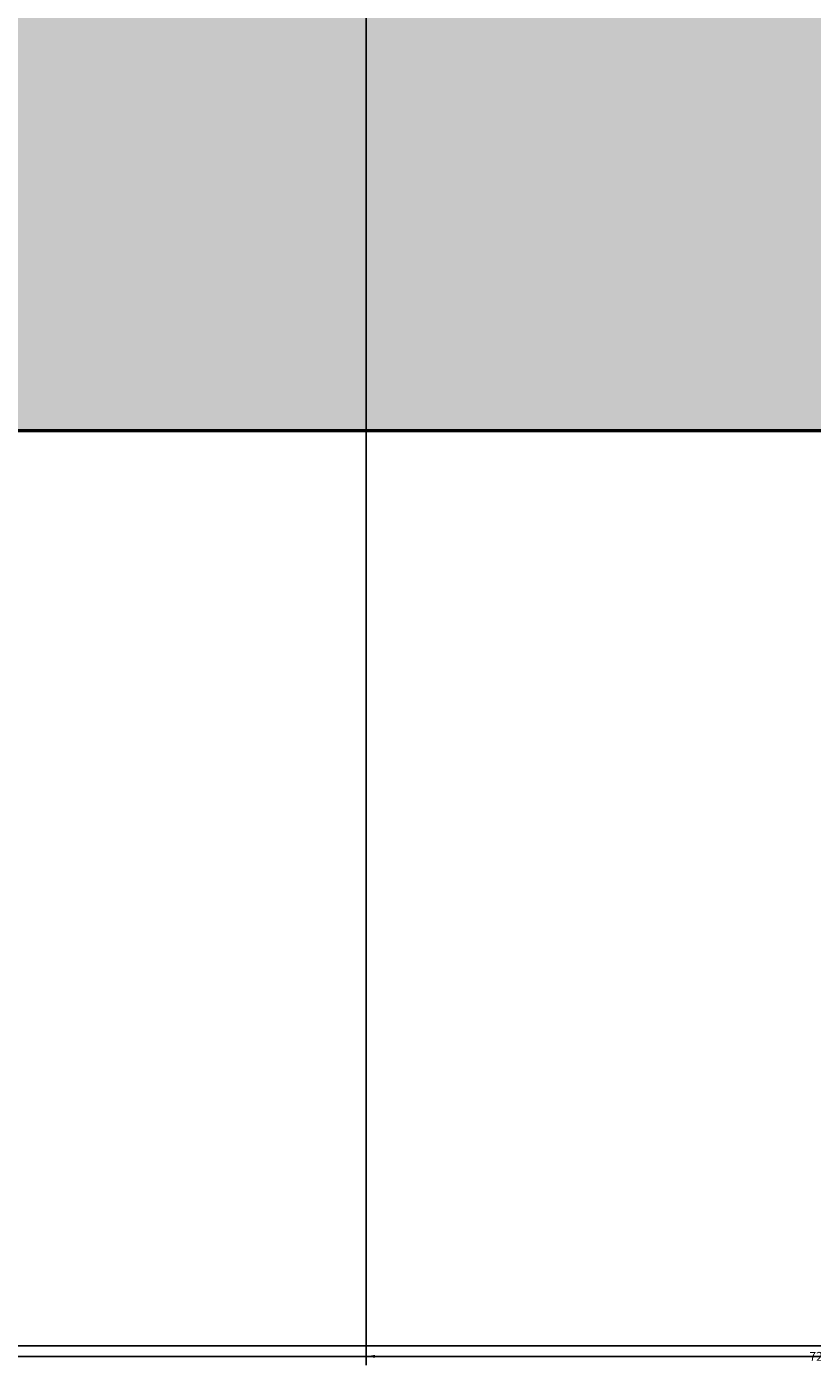
# Model space of a CAD drawing. Units: inches. Extents: x 2231 to 2461, y 2045 to 2455.
# Tile 3 of 95: x 2279 to 2295, y 2045 to 2072. Entities that reach past the tile are written whole.
import ezdxf

# ---------------------------------------------------------------- set-up
doc = ezdxf.new("R2010")
doc.units = ezdxf.units.IN
doc.layers.add('A-ANNO-DIMS', color=2, linetype='Continuous', lineweight=18)
doc.layers.add('A-WALL', color=7, linetype='Continuous', lineweight=50)
doc.layers.add('A-WALL-PATT', color=18, linetype='Continuous', lineweight=13, true_color=0x000000)
doc.styles.get("Standard").update_dxf_attribs({"font": 'arial.ttf'})
doc.dimstyles.get("Standard").update_dxf_attribs({"dimtxt": 0.18, "dimasz": 0.18, "dimexe": 0.18, "dimexo": 0.0625, "dimgap": 0.09, "dimtad": 0, "dimtih": 1, "dimtoh": 1, "dimdec": 4, "dimzin": 0, "dimdsep": 46, "dimtxsty": 'Standard', "dimcen": 0.09, "dimadec": 0, "dimazin": 0, "dimtfac": 1, "dimtdec": 4, "dimtofl": 0, "dimtmove": 0, "dimatfit": 3, "dimfxl": 1, "dimtolj": 1, "dimtzin": 0, "dimarcsym": 0})

# ---------------------------------------------------------------- blocks, each defined once
blk = doc.blocks.new('*D33')
at = {"layer": 'A-ANNO-DIMS', "color": 0, "lineweight": -2, "transparency": 16777216}
for p, q in [((2249.794, 2063.77), (2249.794, 2045.02)), ((2441.794, 2063.77), (2441.794, 2045.02)), ((2249.974, 2045.2), (2345.514, 2045.2)), ((2441.614, 2045.2), (2346.073, 2045.2))]:
    blk.add_line(p, q, dxfattribs=at)
at = {"layer": 'A-ANNO-DIMS', "color": 0, "transparency": 16777216}
for points in [[(2249.974, 2045.23), (2249.974, 2045.17), (2249.794, 2045.2)], [(2441.614, 2045.23), (2441.614, 2045.17), (2441.794, 2045.2)]]:
    blk.add_solid(points, dxfattribs=at)
at = {"layer": 'Defpoints', "color": 0, "transparency": 16777216}
for p in [(2249.794, 2063.833), (2441.794, 2063.833), (2249.794, 2045.2)]:
    blk.add_point(p, dxfattribs=at)
at = {"layer": 'A-ANNO-DIMS', "color": 0, "transparency": 16777216, "insert": (2345.794, 2045.2), "char_height": 0.18, "attachment_point": 5}
blk.add_mtext('\\A1;192', dxfattribs=at)
blk = doc.blocks.new('*D51')
at = {"layer": 'A-ANNO-DIMS', "color": 0, "lineweight": -2, "transparency": 16777216}
for p, q in [((2258.794, 2306.77), (2258.794, 2044.803)), ((2330.794, 2306.77), (2330.794, 2044.803)), ((2258.974, 2044.983), (2294.576, 2044.983)), ((2330.614, 2044.983), (2295.011, 2044.983))]:
    blk.add_line(p, q, dxfattribs=at)
at = {"layer": 'A-ANNO-DIMS', "color": 0, "transparency": 16777216}
for points in [[(2258.974, 2045.013), (2258.974, 2044.953), (2258.794, 2044.983)], [(2330.614, 2045.013), (2330.614, 2044.953), (2330.794, 2044.983)]]:
    blk.add_solid(points, dxfattribs=at)
at = {"layer": 'Defpoints', "color": 0, "transparency": 16777216}
for p in [(2258.794, 2306.833), (2330.794, 2306.833), (2330.794, 2044.983)]:
    blk.add_point(p, dxfattribs=at)
at = {"layer": 'A-ANNO-DIMS', "color": 0, "transparency": 16777216, "insert": (2294.794, 2044.983), "char_height": 0.18, "attachment_point": 5}
blk.add_mtext('\\A1;72', dxfattribs=at)
blk = doc.blocks.new('*D65')
at = {"layer": 'A-ANNO-DIMS', "color": 0, "lineweight": -2, "transparency": 16777216}
for p, q in [((2285.635, 2189.285), (2285.635, 2044.803)), ((2340.667, 2189.285), (2340.667, 2044.803)), ((2285.815, 2044.983), (2312.758, 2044.983)), ((2340.487, 2044.983), (2313.545, 2044.983))]:
    blk.add_line(p, q, dxfattribs=at)
at = {"layer": 'A-ANNO-DIMS', "color": 0, "transparency": 16777216}
for points in [[(2285.815, 2045.013), (2285.815, 2044.953), (2285.635, 2044.983)], [(2340.487, 2045.013), (2340.487, 2044.953), (2340.667, 2044.983)]]:
    blk.add_solid(points, dxfattribs=at)
at = {"layer": 'Defpoints', "color": 0, "transparency": 16777216}
for p in [(2285.635, 2189.348), (2340.667, 2189.348), (2340.667, 2044.983)]:
    blk.add_point(p, dxfattribs=at)
at = {"layer": 'A-ANNO-DIMS', "color": 0, "transparency": 16777216, "insert": (2313.151, 2044.983), "char_height": 0.18, "attachment_point": 5}
blk.add_mtext('\\A1;55.03', dxfattribs=at)

msp = doc.modelspace()

# ---------------------------------------------------------------- hatches: boundary and pattern name
at = {"layer": 'A-WALL-PATT'}
h = msp.add_hatch(color=256, dxfattribs=at)
h.dxf.hatch_style = 1
h.paths.add_polyline_path([(2441.7935, 2269.1535), (2432.7935, 2269.1535), (2432.7935, 2186.8328), (2396.7935, 2186.8328), (2396.7935, 2286.8328), (2394.7935, 2286.8328), (2394.7935, 2186.8328), (2334.7935, 2186.8328), (2334.7935, 2182.8328), (2432.7935, 2182.8328), (2432.7935, 2072.8328), (2416.6639, 2072.8328), (2416.6639, 2063.8328), (2441.7935, 2063.8328)])
h.paths.add_polyline_path([(2368.6639, 2072.8328), (2367.04, 2072.8328), (2330.7942, 2072.8328), (2330.7397, 2063.8328), (2368.6639, 2063.8328)])
h.paths.add_polyline_path([(2300.7392, 2068.3328), (2300.7392, 2072.8328), (2298.7935, 2072.8328), (2294.7935, 2072.8328), (2258.7935, 2072.8328), (2258.7935, 2120.8328), (2294.7935, 2120.8328), (2298.7935, 2120.8328), (2298.7935, 2128.8328), (2294.7935, 2128.8328), (2294.7935, 2124.8328), (2258.7935, 2124.8328), (2258.7935, 2182.8328), (2294.7935, 2182.8328), (2294.7935, 2174.8328), (2298.7935, 2174.8328), (2298.7935, 2182.8328), (2304.7935, 2182.8328), (2304.7935, 2186.8328), (2258.7935, 2186.8328), (2258.7935, 2221.999), (2249.7935, 2221.999), (2249.7935, 2063.8328), (2300.7392, 2063.8328)])
h.paths.add_polyline_path([(2391.9338, 2435.8328), (2333.82, 2435.8328), (2333.82, 2426.8328), (2368.7935, 2426.8328), (2368.7935, 2374.9508), (2368.7935, 2370.8328), (2372.3935, 2370.8328), (2372.7935, 2370.8328), (2372.7935, 2426.8328), (2391.9338, 2426.8328)])
h.paths.add_polyline_path([(2441.7935, 2435.8328), (2415.9338, 2435.8328), (2415.9338, 2426.8328), (2432.7935, 2426.8328), (2432.7935, 2334.8328), (2372.7935, 2334.8328), (2372.7935, 2346.8328), (2368.7935, 2346.8328), (2368.7935, 2306.8328), (2360.7935, 2306.8328), (2360.7935, 2302.8328), (2368.7935, 2302.8328), (2372.7935, 2302.8328), (2372.7935, 2330.8328), (2432.7935, 2330.8328), (2432.7935, 2317.1535), (2441.7935, 2317.1535)])
h.paths.add_polyline_path([(2285.82, 2435.8328), (2249.7935, 2435.8328), (2249.7935, 2269.999), (2258.7935, 2269.999), (2258.7935, 2302.8328), (2318.8168, 2302.8328), (2330.7935, 2302.8328), (2330.7935, 2306.8328), (2258.7935, 2306.8328), (2258.7935, 2426.8328), (2285.82, 2426.8328)])

# ---------------------------------------------------------------- linework, layer by layer
at = {"layer": 'A-WALL'}
msp.add_lwpolyline([(2300.7392, 2063.8328), (2249.7935, 2063.8328), (2249.7935, 2435.8328), (2441.7935, 2435.8328), (2441.7935, 2063.8328), (2330.7397, 2063.8328)], dxfattribs=at)

# ---------------------------------------------------------------- dimensions: what is measured, and where the dimension line sits
at = {"layer": 'A-ANNO-DIMS'}
for base, p1, p2, override, picture, middle in [((2330.7935, 2044.9825), (2258.7935, 2306.8328), (2330.7935, 2306.8328), {"dimdec": 0, "dimlfac": 1, "dimrnd": 0, "dimzin": 0, "dimdsep": 46, "dimlunit": 2}, '*D51', (2294.7935, 2044.9825)), ((2340.6673, 2044.9825), (2285.6353, 2189.3477), (2340.6673, 2189.3477), {"dimdec": 2, "dimlfac": 1, "dimrnd": 0, "dimzin": 0, "dimdsep": 46, "dimlunit": 2}, '*D65', (2313.1513, 2044.9825))]:
    dim = msp.add_linear_dim(base=base, p1=p1, p2=p2, dimstyle='Standard', override=override, dxfattribs=at)
    dim.commit()
    dim.dimension.update_dxf_attribs({"geometry": picture, "text_midpoint": middle})
dim = msp.add_linear_dim(base=(2249.7935, 2045.2003), p1=(2441.7935, 2063.8328), p2=(2249.7935, 2063.8328), angle=180, dimstyle='Standard', override={"dimdec": 0, "dimlfac": 1, "dimrnd": 0, "dimzin": 0, "dimdsep": 46, "dimlunit": 2}, dxfattribs=at)
dim.commit()
dim.dimension.update_dxf_attribs({"geometry": '*D33', "text_midpoint": (2345.7935, 2045.2003)})

doc.saveas('drawing.dxf')
